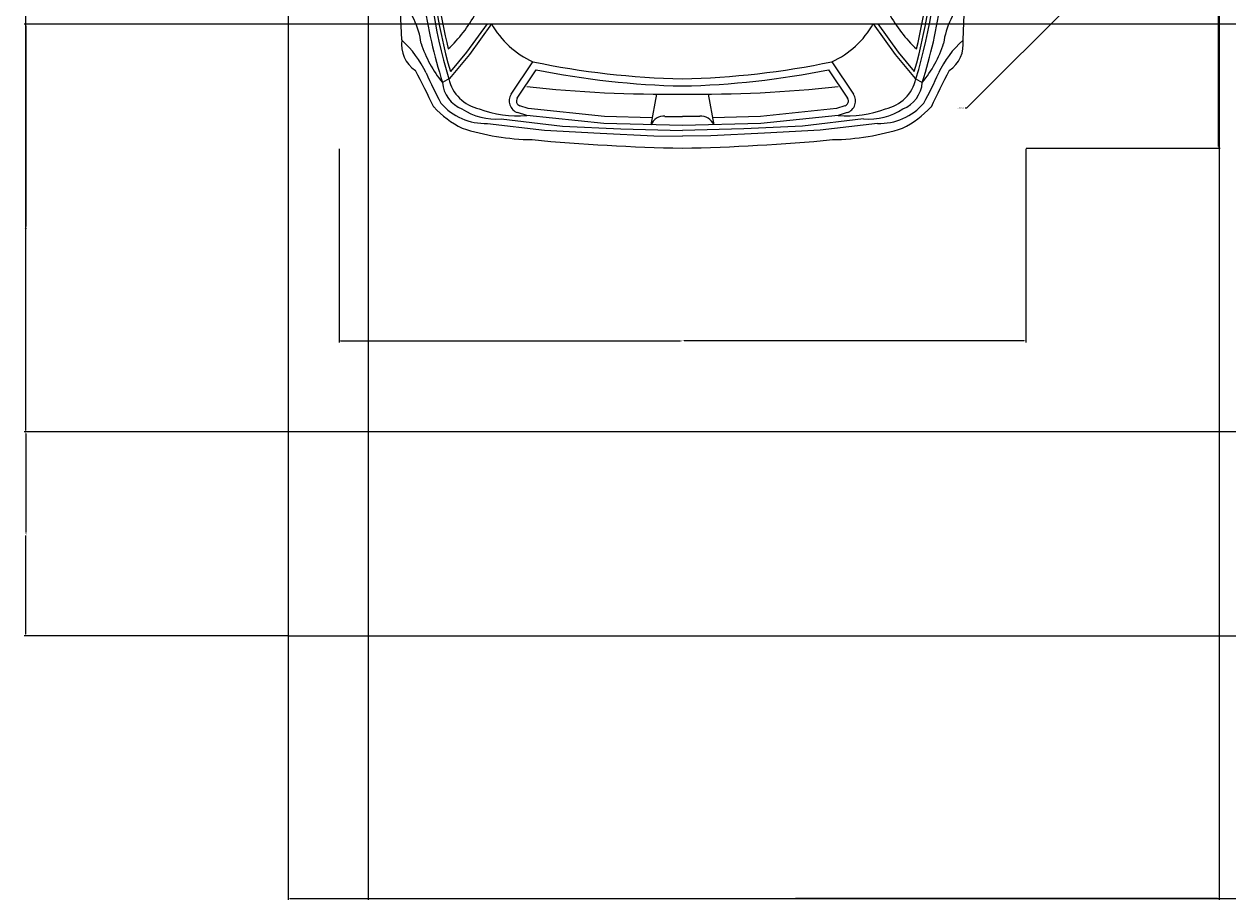
# Model space of a CAD drawing. Units: inches. Extents: x 450 to 1026, y 542 to 1190.
# Tile 1 of 11: x 450 to 586, y 542 to 641. Entities that reach past the tile are written whole.
import ezdxf

# ---------------------------------------------------------------- set-up
doc = ezdxf.new("R2010")
doc.units = ezdxf.units.IN
doc.header["$MEASUREMENT"] = 0
for name, color, linetype, lineweight in [('A-ANNO-DIMS', 2, 'Continuous', 18), ('C-PROP', 7, 'Continuous', 25), ('C-SITE-VEHC', 8, 'Continuous', 13)]:
    doc.layers.add(name, color=color, linetype=linetype, lineweight=lineweight)
doc.styles.get("Standard").update_dxf_attribs({"font": 'arial.ttf'})
doc.dimstyles.get("Standard").update_dxf_attribs({"dimtxt": 0.18, "dimasz": 0.18, "dimexe": 0.18, "dimexo": 0.0625, "dimgap": 0.09, "dimtad": 0, "dimtih": 1, "dimtoh": 1, "dimdec": 4, "dimzin": 0, "dimdsep": 46, "dimtxsty": 'Standard', "dimcen": 0.09, "dimadec": 0, "dimazin": 0, "dimtfac": 1, "dimtdec": 4, "dimtofl": 0, "dimtmove": 0, "dimatfit": 3, "dimfxl": 1, "dimtolj": 1, "dimtzin": 0, "dimarcsym": 0})

# ---------------------------------------------------------------- blocks, each defined once
blk = doc.blocks.new('A$C27D64469')
for p, q in [((-0.7654, -3.667), (-0.7728, -3.5066)), ((0.7926, -3.667), (0.8, -3.5066)), ((-0.5287, -3.6221), (-0.5854, -3.701)), ((-0.5163, -3.6221), (-0.5774, -3.7071)), ((0.5435, -3.6221), (0.6046, -3.7071)), ((0.5559, -3.6221), (0.6126, -3.701)), ((-0.5774, -3.7071), (-0.6331, -3.7742)), ((-0.5854, -3.701), (-0.6302, -3.755)), ((0.6046, -3.7071), (0.6602, -3.7742)), ((0.6126, -3.701), (0.6574, -3.755)), ((-0.4616, -3.818), (-0.4014, -3.7275)), ((0.4285, -3.7275), (0.4887, -3.818)), ((-0.6331, -3.7742), (-0.6525, -3.7849)), ((-0.4449, -3.8291), (-0.3922, -3.7498)), ((0.4193, -3.7498), (0.4721, -3.8291)), ((0.6602, -3.7742), (0.6796, -3.7849)), ((-0.0581, -3.8176), (-0.0735, -3.9028)), ((0.0853, -3.8176), (0.1006, -3.9028)), ((-0.4185, -3.8772), (-0.4442, -3.8686)), ((-0.4142, -3.8575), (-0.4379, -3.8496)), ((-0.2029, -3.8795), (-0.4142, -3.8575)), ((0.4414, -3.8575), (0.2301, -3.8795)), ((0.465, -3.8496), (0.4414, -3.8575)), ((0.4713, -3.8686), (0.4456, -3.8772)), ((-0.5278, -3.8988), (-0.3693, -3.9174)), ((-0.4897, -3.8861), (-0.3195, -3.9066)), ((-0.2042, -3.8994), (-0.4185, -3.8772)), ((-0.3195, -3.9066), (-0.1571, -3.9135)), ((0.0136, -3.905), (-0.2042, -3.8994)), ((-0.0699, -3.8829), (-0.2029, -3.8795)), ((-0.0347, -3.8792), (0.0136, -3.8792)), ((0.0618, -3.8792), (0.0136, -3.8792)), ((0.2314, -3.8994), (0.0136, -3.905)), ((0.2301, -3.8795), (0.097, -3.8829)), ((0.3466, -3.9066), (0.1842, -3.9135)), ((0.4456, -3.8772), (0.2314, -3.8994)), ((0.5168, -3.8861), (0.3466, -3.9066)), ((0.5549, -3.8988), (0.3965, -3.9174)), ((-0.3693, -3.9174), (-0.2148, -3.9262)), ((-0.2148, -3.9262), (-0.0652, -3.933)), ((-0.1571, -3.9135), (0.0136, -3.9184)), ((-0.0652, -3.933), (0.0136, -3.934)), ((0.1842, -3.9135), (0.0136, -3.9184)), ((0.0923, -3.933), (0.0136, -3.934)), ((0.242, -3.9262), (0.0923, -3.933)), ((0.3965, -3.9174), (0.242, -3.9262))]:
    blk.add_line(p, q)
for centre, radius, start, end in [((0.8768, -3.3275), 1.5766, 180.7904, 196.499), ((0.8768, -3.3275), 1.5665, 180.7904, 195.8378), ((-0.8496, -3.3275), 1.5665, 344.1622, 359.2096), ((-0.8496, -3.3275), 1.5766, 343.501, 359.2096), ((0.8768, -3.3275), 1.5564, 182.4426, 193.5531), ((-0.8496, -3.3275), 1.5564, 346.4469, 357.5574), ((-0.931, -3.7054), 0.2213, 7.498, 43.5729), ((0.6722, -3.364), 1.3899, 187.9913, 197.6257), ((-0.645, -3.364), 1.3899, 342.3743, 352.0087), ((0.9581, -3.7054), 0.2213, 136.4271, 172.502), ((-0.9014, -3.4088), 0.388, 313.0938, 331.4872), ((0.9285, -3.4088), 0.388, 208.5128, 226.9062), ((-0.3005, -3.502), 0.247, 209.0915, 245.8956), ((0.3276, -3.502), 0.247, 294.1044, 330.9085), ((-0.6785, -3.679), 0.0877, 172.132, 236.2396), ((-0.9429, -3.8711), 0.2695, 24.6265, 48.8595), ((0.97, -3.8711), 0.2695, 131.1405, 155.3735), ((0.7057, -3.679), 0.0877, 303.7604, 7.868), ((-0.3962, -3.5747), 0.3315, 197.8909, 219.3552), ((0.4233, -3.5747), 0.3315, 320.6448, 342.1091), ((0.0567, -1.5526), 2.2226, 258.1061, 268.8881), ((-0.0296, -1.5526), 2.2226, 271.1119, 281.8939), ((-3.375, -5.1387), 2.9889, 25.4724, 27.6425), ((0.5567, -3.1915), 1.3769, 204.3314, 208.2014), ((-0.528, -3.7506), 0.1097, 192.9436, 258.3207), ((0.0567, -1.5526), 2.2426, 258.453, 268.898), ((-0.0296, -1.5526), 2.2426, 271.102, 281.547), ((0.5551, -3.7506), 0.1097, 281.6793, 347.0564), ((-0.5295, -3.1915), 1.3769, 331.7986, 335.6686), ((3.4021, -5.1387), 2.9889, 152.3575, 154.5276), ((-0.566, -3.7782), 0.0867, 184.4324, 248.21), ((-0.0346, -0.3333), 3.4843, 263.6749, 270.7924), ((0.0618, -0.3333), 3.4843, 269.2076, 276.3251), ((0.5932, -3.7782), 0.0867, 291.79, 355.5676), ((-0.5341, -3.738), 0.1609, 220.3568, 272.2613), ((-0.4335, -3.8367), 0.0337, 146.3764, 251.5583), ((-0.4335, -3.8367), 0.0137, 146.3764, 251.5583), ((0.4607, -3.8367), 0.0137, 288.4417, 33.6236), ((0.4607, -3.8367), 0.0337, 288.4417, 33.6236), ((0.5613, -3.738), 0.1609, 267.7387, 319.6432), ((-0.4633, -3.6496), 0.2949, 223.6549, 242.8613), ((-0.5047, -3.7168), 0.17, 236.6049, 275.0704), ((-0.4436, -3.5867), 0.2916, 248.5479, 274.9353), ((0.4707, -3.5867), 0.2916, 265.0647, 291.4521), ((0.5318, -3.7168), 0.17, 264.9296, 303.3951), ((0.4904, -3.6496), 0.2949, 297.1387, 316.3451), ((-0.0379, -3.9176), 0.0386, 85.1824, 157.357), ((0.065, -3.9176), 0.0386, 22.643, 94.8176), ((-0.3932, -3.2709), 0.673, 252.2974, 269.1096), ((0.4203, -3.2709), 0.673, 270.8904, 287.7026), ((0.1171, 1.5736), 5.542, 264.6089, 268.93), ((-0.0899, 1.5736), 5.542, 271.07, 275.3911)]:
    blk.add_arc(centre, radius, start, end)
blk = doc.blocks.new('*D43')
at = {"layer": 'A-ANNO-DIMS', "color": 0, "lineweight": -2, "transparency": 16777216}
for p, q in [((562.89, 771.86), (584.74, 771.86)), ((584.56, 771.68), (584.56, 699.59)), ((584.56, 627.13), (584.56, 699.22)), ((562.89, 626.95), (584.74, 626.95))]:
    blk.add_line(p, q, dxfattribs=at)
at = {"layer": 'A-ANNO-DIMS', "color": 0, "transparency": 16777216}
for points in [[(584.53, 771.68), (584.59, 771.68), (584.56, 771.86)], [(584.53, 627.13), (584.59, 627.13), (584.56, 626.95)]]:
    blk.add_solid(points, dxfattribs=at)
at = {"layer": 'Defpoints', "color": 0, "transparency": 16777216}
for p in [(562.83, 771.86), (584.56, 771.86), (562.83, 626.95)]:
    blk.add_point(p, dxfattribs=at)
at = {"layer": 'A-ANNO-DIMS', "color": 0, "transparency": 16777216, "insert": (584.56, 699.41), "char_height": 0.18, "attachment_point": 5}
blk.add_mtext('\\A1;VEHICLE 145', dxfattribs=at)
blk = doc.blocks.new('*D44')
at = {"layer": 'A-ANNO-DIMS', "color": 0, "lineweight": -2, "transparency": 16777216}
for p, q in [((485.37, 626.89), (485.37, 605.03)), ((562.83, 626.89), (562.83, 605.03)), ((485.55, 605.21), (523.88, 605.21)), ((562.65, 605.21), (524.31, 605.21))]:
    blk.add_line(p, q, dxfattribs=at)
at = {"layer": 'A-ANNO-DIMS', "color": 0, "transparency": 16777216}
for points in [[(485.55, 605.24), (485.55, 605.18), (485.37, 605.21)], [(562.65, 605.24), (562.65, 605.18), (562.83, 605.21)]]:
    blk.add_solid(points, dxfattribs=at)
at = {"layer": 'Defpoints', "color": 0, "transparency": 16777216}
for p in [(485.37, 626.95), (562.83, 626.95), (562.83, 605.21)]:
    blk.add_point(p, dxfattribs=at)
at = {"layer": 'A-ANNO-DIMS', "color": 0, "transparency": 16777216, "insert": (524.1, 605.21), "char_height": 0.18, "attachment_point": 5}
blk.add_mtext('\\A1;77', dxfattribs=at)
blk = doc.blocks.new('*D45')
at = {"layer": 'A-ANNO-DIMS', "color": 0, "lineweight": -2, "transparency": 16777216}
for p, q in [((479.65, 571.88), (479.65, 542.16)), ((995.65, 571.88), (995.65, 542.16)), ((479.83, 542.34), (737.36, 542.34)), ((995.47, 542.34), (737.94, 542.34))]:
    blk.add_line(p, q, dxfattribs=at)
at = {"layer": 'A-ANNO-DIMS', "color": 0, "transparency": 16777216}
for points in [[(479.83, 542.37), (479.83, 542.31), (479.65, 542.34)], [(995.47, 542.37), (995.47, 542.31), (995.65, 542.34)]]:
    blk.add_solid(points, dxfattribs=at)
at = {"layer": 'Defpoints', "color": 0, "transparency": 16777216}
for p in [(479.65, 571.94), (995.65, 571.94), (995.65, 542.34)]:
    blk.add_point(p, dxfattribs=at)
at = {"layer": 'A-ANNO-DIMS', "color": 0, "transparency": 16777216, "insert": (737.65, 542.34), "char_height": 0.18, "attachment_point": 5}
blk.add_mtext('\\A1;516', dxfattribs=at)
blk = doc.blocks.new('*D53')
at = {"layer": 'A-ANNO-DIMS', "color": 0, "lineweight": -2, "transparency": 16777216}
for p, q in [((479.59, 817.94), (449.87, 817.94)), ((450.05, 817.76), (450.05, 706.62)), ((450.05, 595.12), (450.05, 706.26)), ((797.59, 594.94), (449.87, 594.94))]:
    blk.add_line(p, q, dxfattribs=at)
at = {"layer": 'A-ANNO-DIMS', "color": 0, "transparency": 16777216}
for points in [[(450.02, 817.76), (450.08, 817.76), (450.05, 817.94)], [(450.02, 595.12), (450.08, 595.12), (450.05, 594.94)]]:
    blk.add_solid(points, dxfattribs=at)
at = {"layer": 'Defpoints', "color": 0, "transparency": 16777216}
for p in [(479.65, 817.94), (450.05, 594.94), (797.65, 594.94)]:
    blk.add_point(p, dxfattribs=at)
at = {"layer": 'A-ANNO-DIMS', "color": 0, "transparency": 16777216, "insert": (450.05, 706.44), "char_height": 0.18, "attachment_point": 5}
blk.add_mtext('\\A1;223', dxfattribs=at)
blk = doc.blocks.new('*D54')
at = {"layer": 'A-ANNO-DIMS', "color": 0, "lineweight": -2, "transparency": 16777216}
for p, q in [((797.59, 594.94), (449.87, 594.94)), ((450.05, 594.76), (450.05, 583.62)), ((450.05, 572.12), (450.05, 583.26)), ((479.59, 571.94), (449.87, 571.94))]:
    blk.add_line(p, q, dxfattribs=at)
at = {"layer": 'A-ANNO-DIMS', "color": 0, "transparency": 16777216}
for points in [[(450.02, 594.76), (450.08, 594.76), (450.05, 594.94)], [(450.02, 572.12), (450.08, 572.12), (450.05, 571.94)]]:
    blk.add_solid(points, dxfattribs=at)
at = {"layer": 'Defpoints', "color": 0, "transparency": 16777216}
for p in [(797.65, 594.94), (450.05, 571.94), (479.65, 571.94)]:
    blk.add_point(p, dxfattribs=at)
at = {"layer": 'A-ANNO-DIMS', "color": 0, "transparency": 16777216, "insert": (450.05, 583.44), "char_height": 0.18, "attachment_point": 5}
blk.add_mtext('\\A1;23', dxfattribs=at)
blk = doc.blocks.new('*D56')
at = {"layer": 'A-ANNO-DIMS', "color": 0, "lineweight": -2, "transparency": 16777216}
for p, q in [((488.65, 1150.88), (488.65, 542.16)), ((584.65, 1150.88), (584.65, 542.16)), ((488.83, 542.34), (536.43, 542.34)), ((584.47, 542.34), (536.87, 542.34))]:
    blk.add_line(p, q, dxfattribs=at)
at = {"layer": 'A-ANNO-DIMS', "color": 0, "transparency": 16777216}
for points in [[(488.83, 542.37), (488.83, 542.31), (488.65, 542.34)], [(584.47, 542.37), (584.47, 542.31), (584.65, 542.34)]]:
    blk.add_solid(points, dxfattribs=at)
at = {"layer": 'Defpoints', "color": 0, "transparency": 16777216}
for p in [(488.65, 1150.94), (584.65, 1150.94), (584.65, 542.34)]:
    blk.add_point(p, dxfattribs=at)
at = {"layer": 'A-ANNO-DIMS', "color": 0, "transparency": 16777216, "insert": (536.65, 542.34), "char_height": 0.18, "attachment_point": 5}
blk.add_mtext('\\A1;96', dxfattribs=at)
blk = doc.blocks.new('*D73')
at = {"layer": 'A-ANNO-DIMS', "color": 0, "lineweight": -2, "transparency": 16777216}
for p, q in [((797.59, 640.94), (449.87, 640.94)), ((450.05, 640.76), (450.05, 618.12)), ((450.05, 595.12), (450.05, 617.76)), ((797.59, 594.94), (449.87, 594.94))]:
    blk.add_line(p, q, dxfattribs=at)
at = {"layer": 'A-ANNO-DIMS', "color": 0, "transparency": 16777216}
for points in [[(450.02, 640.76), (450.08, 640.76), (450.05, 640.94)], [(450.02, 595.12), (450.08, 595.12), (450.05, 594.94)]]:
    blk.add_solid(points, dxfattribs=at)
at = {"layer": 'Defpoints', "color": 0, "transparency": 16777216}
for p in [(450.05, 640.94), (797.65, 640.94), (797.65, 594.94)]:
    blk.add_point(p, dxfattribs=at)
at = {"layer": 'A-ANNO-DIMS', "color": 0, "transparency": 16777216, "insert": (450.05, 617.94), "char_height": 0.18, "attachment_point": 5}
blk.add_mtext('\\A1;46', dxfattribs=at)
blk = doc.blocks.new('*D75')
at = {"layer": 'A-ANNO-DIMS', "color": 0, "lineweight": -2, "transparency": 16777216}
for p, q in [((637.56, 712.94), (637.74, 712.94)), ((637.65, 712.85), (637.65, 713.03)), ((556.19, 631.48), (586.61, 661.9)), ((556.01, 631.48), (556.19, 631.48))]:
    blk.add_line(p, q, dxfattribs=at)
at = {"layer": 'A-ANNO-DIMS', "color": 0, "transparency": 16777216}
blk.add_solid([(586.59, 661.92), (586.63, 661.88), (586.74, 662.03)], dxfattribs=at)
at = {"layer": 'Defpoints', "color": 0, "transparency": 16777216}
for p in [(637.65, 712.94), (586.74, 662.03)]:
    blk.add_point(p, dxfattribs=at)
at = {"layer": 'A-ANNO-DIMS', "color": 0, "transparency": 16777216, "insert": (555.51, 631.48), "char_height": 0.18, "attachment_point": 5}
blk.add_mtext('\\A1;2X R72', dxfattribs=at)

msp = doc.modelspace()

# ---------------------------------------------------------------- linework, layer by layer
at = {"layer": 'C-PROP'}
for p, q in [((479.6513, 1159.9426), (479.6513, 571.9426)), ((479.6513, 571.9426), (995.6513, 571.9426))]:
    msp.add_line(p, q, dxfattribs=at)

# ---------------------------------------------------------------- block references
at = {"layer": 'C-SITE-VEHC', "xscale": 40.63350989877505, "yscale": 40.63350989877505, "zscale": 40.63350989877505}
msp.add_blockref('A$C27D64469', (523.5448, 788.1608), dxfattribs=at)

# ---------------------------------------------------------------- dimensions: what is measured, and where the dimension line sits
at = {"layer": 'A-ANNO-DIMS'}
for base, p1, p2, picture, middle in [((584.6513, 542.3426), (488.6513, 1150.9426), (584.6513, 1150.9426), '*D56', (536.6513, 542.3426)), ((562.8259, 605.2135), (485.3667, 626.9507), (562.8259, 626.9507), '*D44', (524.0963, 605.2135)), ((995.6513, 542.3426), (479.6513, 571.9426), (995.6513, 571.9426), '*D45', (737.6513, 542.3426))]:
    dim = msp.add_linear_dim(base=base, p1=p1, p2=p2, dimstyle='Standard', override={"dimdec": 0, "dimlfac": 1, "dimrnd": 0, "dimzin": 0, "dimdsep": 46, "dimlunit": 2}, dxfattribs=at)
    dim.commit()
    dim.dimension.update_dxf_attribs({"geometry": picture, "text_midpoint": middle})
for base, p1, p2, picture, middle in [((450.0513, 594.9426), (479.6513, 817.9426), (797.6513, 594.9426), '*D53', (450.0513, 706.4426)), ((450.0513, 640.9426), (797.6513, 594.9426), (797.6513, 640.9426), '*D73', (450.0513, 617.9426)), ((450.0513, 571.9426), (797.6513, 594.9426), (479.6513, 571.9426), '*D54', (450.0513, 583.4426))]:
    dim = msp.add_linear_dim(base=base, p1=p1, p2=p2, angle=90, dimstyle='Standard', override={"dimdec": 0, "dimlfac": 1, "dimrnd": 0, "dimzin": 0, "dimdsep": 46, "dimlunit": 2}, dxfattribs=at)
    dim.commit()
    dim.dimension.update_dxf_attribs({"geometry": picture, "text_midpoint": middle})
dim = msp.add_linear_dim(base=(584.563, 771.8648), p1=(562.8259, 626.9507), p2=(562.8259, 771.8648), angle=90, text='VEHICLE <>', dimstyle='Standard', override={"dimdec": 0, "dimlfac": 1, "dimrnd": 0, "dimzin": 0, "dimdsep": 46, "dimlunit": 2}, dxfattribs=at)
dim.commit()
dim.dimension.update_dxf_attribs({"geometry": '*D43', "text_midpoint": (584.563, 699.4077)})
dim = msp.add_radius_dim(center=(637.6513, 712.9426), mpoint=(586.7403, 662.0303), text='2X <>', dimstyle='Standard', override={"dimdec": 0, "dimlfac": 1, "dimrnd": 0, "dimzin": 0, "dimdsep": 46, "dimlunit": 2}, dxfattribs=at)
dim.commit()
dim.dimension.update_dxf_attribs({"geometry": '*D75', "text_midpoint": (555.5146, 631.4829), "dimtype": 164})

doc.saveas('drawing.dxf')
